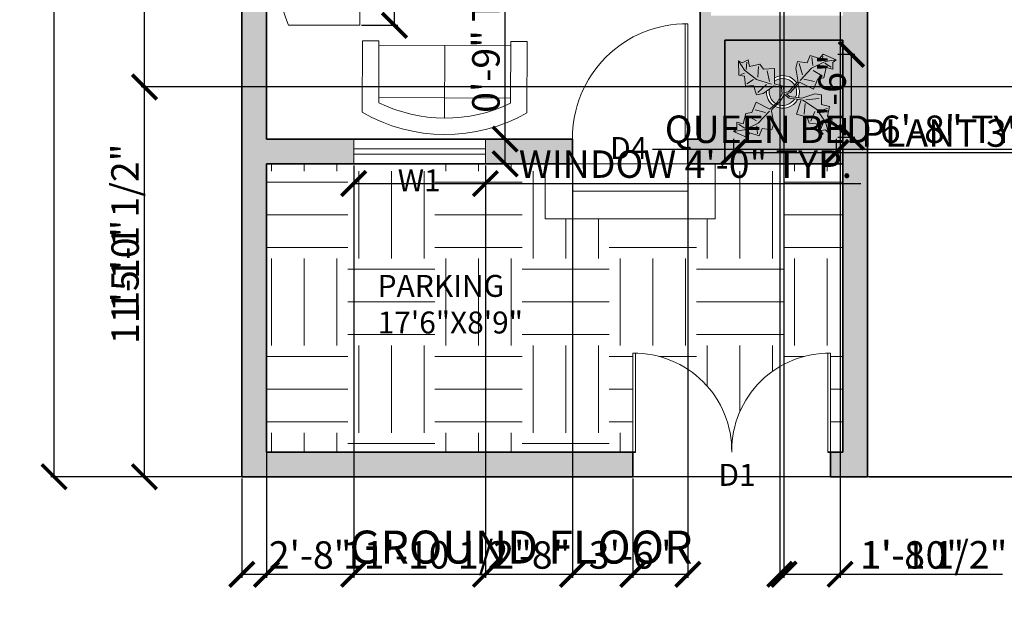
# Model space of a CAD drawing. Units: inches. Extents: x 2570 to 3313, y 1387 to 2106.
# Tile 1 of 5: x 2579 to 2938, y 1396 to 1607. Entities that reach past the tile are written whole.
import ezdxf

# ---------------------------------------------------------------- set-up
doc = ezdxf.new("R2010")
doc.units = ezdxf.units.IN
for name, color, linetype, lineweight in [('A-ANNO-DIMS', 7, 'Continuous', 18), ('DOORS', 195, 'Continuous', 18), ('furniture', 11, 'Continuous', 18), ('PLANT', 107, 'Continuous', 18), ('STAIRS', 13, 'Continuous', 18), ('WALLS', 20, 'Continuous', 35), ('WINDOWS', 15, 'Continuous', 18)]:
    doc.layers.add(name, color=color, linetype=linetype, lineweight=lineweight)
for name, color, linetype, lineweight, true_color in [('A-ANNO-TEXT', 143, 'Continuous', 18, 0x7aafdf), ('A-ANNO-TITL', 52, 'Continuous', 25, 0xc8c92d), ('A-AREA-IDEN', 143, 'Continuous', 18, 0x7aafdf), ('A-FLOR-PATT', 254, 'Continuous', 13, 0xcecce6), ('A-WALL-PATT', 30, 'Continuous', 13, 0xf26722), ('L-PLNT-PATT', 114, 'Continuous', 13, 0x139b48)]:
    doc.layers.add(name, color=color, linetype=linetype, lineweight=lineweight, true_color=true_color)
doc.styles.get("Standard").update_dxf_attribs({"font": 'arial.ttf'})
doc.dimstyles.new('ISO-25', dxfattribs={"dimtxt": 10, "dimasz": 9, "dimexe": 1.25, "dimexo": 0.625, "dimtad": 1, "dimdec": 0, "dimlunit": 3, "dimtxsty": 'Standard', "dimblk": 'ARCHTICK', "dimcen": 2.5, "dimadec": 0, "dimazin": 0, "dimtfac": 1, "dimtdec": 0, "dimtmove": 0, "dimatfit": 3, "dimfxl": 1, "dimarcsym": 0})

# ---------------------------------------------------------------- blocks, each defined once
blk = doc.blocks.new('Plant - Rubber or Philodendron')
for p, q in [((-16.2005, 11.4774), (-13.9899, 8.1064)), ((-16.2005, 11.4774), (-14.8639, 10.7964)), ((-16.0159, 6.3329), (-16.2005, 11.4774)), ((-14.8639, 10.7964), (-12.6195, 11.8975)), ((-13.3174, 8.325), (-13.0735, 11.0065)), ((-12.6195, 11.8975), (-12.1909, 9.4345)), ((4.6914, 8.8812), (5.3859, 11.2828)), ((5.3859, 11.2828), (8.8871, 10.7908)), ((8.8871, 10.7908), (9.9809, 13.4933)), ((9.9809, 13.4933), (13.3837, 12.301)), ((15.3859, 11.3055), (10.3916, 8.7942)), ((10.5828, 12.6946), (10.8893, 9.7953)), ((13.3837, 12.301), (14.68, 13.9039)), ((14.5816, 13.2037), (14.3848, 11.8033)), ((14.68, 13.9039), (19.3848, 11.8146)), ((19.3848, 11.8146), (15.3859, 11.3055)), ((19.3848, 11.8146), (18.1868, 10.9119)), ((18.1868, 10.9119), (18.1925, 8.4119)), ((-13.9899, 8.1064), (-9.5434, 4.7185)), ((-12.1909, 9.4345), (-8.3829, 10.3)), ((-8.8369, 9.409), (-9.0894, 5.6095)), ((-8.3829, 10.3), (-7.0549, 8.501)), ((-7.0549, 8.501), (-3.0284, 8.6941)), ((-4.8529, 4.012), (-5.7184, 7.82)), ((-3.0284, 8.6941), (-3.0709, 3.1041)), ((4.6914, 8.8812), (5.5014, 4.4831)), ((5.9878, 10.4842), (7.1971, 6.3869)), ((10.3916, 8.7942), (6.2847, 4.4028)), ((14.2977, 6.1031), (10.9934, 7.9956)), ((15.7909, 9.1065), (14.8995, 5.3044)), ((15.2875, 10.6053), (17.5907, 9.2105)), ((18.1925, 8.4119), (15.7909, 9.1065)), ((-14.0069, 5.8704), (-16.0159, 6.3329)), ((-15.3434, 6.5514), (-13.9984, 6.9884)), ((-13.5868, 2.2894), (-14.0069, 5.8704)), ((-13.1329, 3.1804), (-10.6614, 4.727)), ((-9.5434, 4.7185), (-4.1917, 2.9888)), ((2.1141, 0.2298), (5.4346, 3.9146)), ((6.1032, 3.6844), (2.8262, -0.031)), ((5.4346, 3.9146), (5.5014, 4.4831)), ((11.1089, 1.1958), (6.1032, 3.6844)), ((7.7005, 4.8881), (11.5025, 3.9967)), ((12.7005, 4.8994), (11.1089, 1.1958)), ((14.8995, 5.3044), (12.7005, 4.8994)), ((-10.6784, 2.491), (-13.5868, 2.2894)), ((-9.5858, -0.8715), (-10.6784, 2.491)), ((-9.1318, 0.0195), (-5.9793, 2.9025)), ((-7.1228, -0.443), (-3.5248, 2.2131)), ((-3.5248, 2.2131), (-3.3011, 2.4355)), ((-3.3011, 2.4355), (-0.5306, 1.7947)), ((-3.0709, 3.1041), (0.0797, 2.3163)), ((-0.5306, 1.7947), (-0.2255, -0.5527)), ((-0.5306, 1.7947), (-0.5306, 1.7947)), ((0.0797, 2.3163), (0.4866, -0.031)), ((0.4866, -0.031), (2.1141, 0.2298)), ((-11.3237, -7.2629), (-9.7321, -3.5593)), ((-9.7321, -3.5593), (-4.7264, -6.0479)), ((-7.1228, -0.443), (-9.5858, -0.8715)), ((-4.0579, -6.2781), (-0.9375, -3.1608)), ((-2.019, -3.6148), (-0.2255, -0.5527)), ((-0.9375, -3.1608), (0.5883, -0.8135)), ((0.5883, -0.8135), (2.2447, -2.0916)), ((2.8262, -0.031), (1.3003, -0.5527)), ((1.3003, -0.5527), (2.4193, -1.4655)), ((2.2447, -2.0916), (6.7108, -2.6626)), ((2.4193, -1.4655), (6.895, -2.1175)), ((4.943, -7.9659), (6.7108, -2.6626)), ((11.6605, -0.5413), (6.895, -2.1175)), ((12.3677, -6.1981), (7.219, -2.6772)), ((8.3544, -2.7453), (13.1973, -2.1704)), ((11.6605, -0.5413), (14.1354, -0.8948)), ((14.1354, -0.8948), (14.1354, -4.4304)), ((-6.3237, -7.2516), (-10.1257, -6.3602)), ((-9.0148, -11.1577), (-4.9047, -6.8122)), ((-2.019, -3.6148), (-4.7264, -6.0479)), ((-4.1246, -6.8466), (-4.0579, -6.2781)), ((-3.3146, -11.2447), (-4.1246, -6.8466)), ((8.125, -4.0768), (7.7715, -7.9659)), ((10.2463, -10.4408), (11.6605, -6.9053)), ((15.5496, -10.7943), (12.3677, -6.1981)), ((16.2567, -5.8446), (13.4283, -6.5517)), ((14.1354, -4.4304), (16.9638, -5.1375)), ((16.9638, -5.1375), (16.2567, -8.673)), ((-14.4141, -11.4699), (-13.5228, -7.6679)), ((-13.5228, -7.6679), (-11.3237, -7.2629)), ((-12.921, -8.4665), (-9.6166, -10.359)), ((-4.611, -12.8477), (-5.8203, -8.7504)), ((8.8321, -9.0266), (4.943, -7.9659)), ((9.5392, -11.1479), (8.8321, -9.0266)), ((17.3174, -9.7337), (15.9032, -9.7337)), ((16.2567, -8.673), (18.0245, -9.7337)), ((18.0245, -9.7337), (16.6103, -14.6834)), ((-18.008, -14.1781), (-16.8101, -13.2754)), ((-18.008, -14.1781), (-14.0091, -13.669)), ((-13.3032, -16.2674), (-18.008, -14.1781)), ((-16.8157, -10.7754), (-14.4141, -11.4699)), ((-16.8101, -13.2754), (-16.8157, -10.7754)), ((-13.9107, -12.9688), (-16.2139, -11.574)), ((-14.0091, -13.669), (-9.0148, -11.1577)), ((-13.2048, -15.5672), (-13.008, -14.1668)), ((-9.206, -15.0581), (-9.5126, -12.1588)), ((-7.5103, -13.1543), (-8.6042, -15.8568)), ((-4.0092, -13.6463), (-7.5103, -13.1543)), ((-3.3146, -11.2447), (-4.0092, -13.6463)), ((13.4283, -11.5015), (9.5392, -11.1479)), ((13.0748, -13.9763), (13.4283, -11.5015)), ((15.5496, -13.6228), (13.0748, -13.9763)), ((14.8425, -10.7943), (13.7819, -13.2692)), ((16.6103, -14.6834), (15.5496, -10.7943)), ((16.6103, -14.6834), (15.5496, -13.6228)), ((-12.0069, -14.6645), (-13.3032, -16.2674)), ((-8.6042, -15.8568), (-12.0069, -14.6645))]:
    blk.add_line(p, q)
for centre, radius, start, end in [((0, 0), 6.1275, 34.37569, 120.1028), ((-0.0601, -0.2075), 5.2461, 33.82192, 124.9414), ((0.0308, 0.1664), 6, 178.6147, 235.1169), ((0.0308, 0.1664), 5, 168.1647, 238.6725), ((-0.2664, 0.1682), 5.2775, 338.4094, 20.03007), ((-0.098, 0.1364), 6.1288, 341.2017, 26.09184), ((-0.0234, 0.3825), 6.1492, 242.5812, 331.2714), ((-0.1102, 0.4886), 5.2883, 247.3711, 327.472)]:
    blk.add_arc(centre, radius, start, end)
blk = doc.blocks.new('Sofa - Roundback 7 ft.')
for p, q in [((-12.00002, -32.4421), (-12.00003, -6.5971)), ((11.99997, -32.4421), (11.99998, -6.5971)), ((-36.000027, -34), (-36.000027, -11.4696)), ((-35.999844, -13.3819), (35.9998, -13.3819)), ((35.99998, -34), (35.99998, -11.4696)), ((-36.000027, -32.4421), (35.99998, -32.4421))]:
    blk.add_line(p, q)
for points in [[(-36.000027, -34), (-42.000027, -34), (-42.000027, -8)], [(41.99998, -8), (41.99998, -34), (35.99998, -34)]]:
    blk.add_lwpolyline(points)
for centre, radius, start, end in [((0, -114.25), 114.25, 68.43141, 111.5686), ((-0.00001, -127.1968), 121.1968, 72.72033, 107.2797)]:
    blk.add_arc(centre, radius, start, end)
blk = doc.blocks.new('Sofa - Roundback Loveseat 5 ft.')
for p, q in [((0, -32.44198), (0, -5.99998)), ((-24, -33.99998), (-24, -11.46958)), ((-23.9998, -13.38178), (23.99986, -13.38178)), ((24.00004, -33.99998), (24.00004, -11.46958)), ((-24, -32.44198), (24.00004, -32.44198))]:
    blk.add_line(p, q)
for points in [[(-24, -33.99998), (-30, -33.99998), (-30, -7.99998)], [(30.00004, -7.99998), (30.00004, -33.99998), (24.00004, -33.99998)]]:
    blk.add_lwpolyline(points)
for centre, radius, start, end in [((0, -60.24998), 60.24998, 60.13715, 119.8628), ((0, -61.38438), 55.38444, 64.32083, 115.6792)]:
    blk.add_arc(centre, radius, start, end)
blk = doc.blocks.new('_ArchTick')
at = {"color": 0, "linetype": 'ByBlock', "const_width": 0.15}
blk.add_lwpolyline([(-0.5, -0.5), (0.5, 0.5)], dxfattribs=at)
blk = doc.blocks.new('*D20')
at = {"layer": 'A-ANNO-DIMS', "color": 0, "lineweight": -2, "transparency": 16777216}
for p, q in [((2659.53, 2040.49), (2590.49, 2040.49)), ((2591.74, 1440.49), (2591.74, 2040.49)), ((2659.53, 1440.49), (2590.49, 1440.49))]:
    blk.add_line(p, q, dxfattribs=at)
at = {"layer": 'Defpoints', "color": 0, "transparency": 16777216}
for p in [(2591.74, 2040.49), (2660.15, 2040.49), (2660.15, 1440.49)]:
    blk.add_point(p, dxfattribs=at)
at = {"layer": 'A-ANNO-DIMS', "color": 0, "lineweight": -2, "transparency": 16777216, "xscale": 9, "yscale": 9, "zscale": 9}
for p, rotation in [((2591.74, 2040.49), 90), ((2591.74, 1440.49), 270)]:
    blk.add_blockref('_ArchTick', p, dxfattribs=dict(at, rotation=rotation))
at = {"layer": 'A-ANNO-DIMS', "color": 0, "transparency": 16777216, "insert": (2586.01, 1740.49), "char_height": 10, "attachment_point": 5, "rotation": 90}
blk.add_mtext("50'", dxfattribs=at)
blk = doc.blocks.new('WIN-48IN')
for p, q in [((-48, 0), (-48, -9)), ((0, 0), (0, -9)), ((0, -3.5), (-48, -3.5)), ((0, -5.5), (-48, -5.5))]:
    blk.add_line(p, q)
blk = doc.blocks.new('*D37')
at = {"layer": 'A-ANNO-DIMS', "color": 0, "lineweight": -2, "transparency": 16777216}
for p, q in [((2700.9, 1553.86), (2700.9, 1546.04)), ((2748.9, 1553.86), (2748.9, 1546.04)), ((2700.9, 1547.29), (2748.9, 1547.29)), ((2748.9, 1547.29), (2885.7, 1547.29))]:
    blk.add_line(p, q, dxfattribs=at)
at = {"layer": 'Defpoints', "color": 0, "transparency": 16777216}
for p in [(2700.9, 1554.49), (2748.9, 1554.49), (2748.9, 1547.29)]:
    blk.add_point(p, dxfattribs=at)
at = {"layer": 'A-ANNO-DIMS', "color": 0, "lineweight": -2, "transparency": 16777216, "xscale": 9, "yscale": 9, "zscale": 9, "rotation": 180}
blk.add_blockref('_ArchTick', (2700.9, 1547.29), dxfattribs=at)
at = {"layer": 'A-ANNO-DIMS', "color": 0, "lineweight": -2, "transparency": 16777216, "xscale": 9, "yscale": 9, "zscale": 9}
blk.add_blockref('_ArchTick', (2748.9, 1547.29), dxfattribs=at)
at = {"layer": 'A-ANNO-DIMS', "color": 0, "transparency": 16777216, "insert": (2821.8, 1553.09), "char_height": 10, "attachment_point": 5}
blk.add_mtext('WINDOW 4\'-0" TYP.', dxfattribs=at)
blk = doc.blocks.new('*D38')
at = {"layer": 'A-ANNO-DIMS', "color": 0, "lineweight": -2, "transparency": 16777216}
for p, q in [((2756.1, 1563.49), (2756.1, 1634.69)), ((2749.53, 1563.49), (2757.35, 1563.49)), ((2756.1, 1554.49), (2756.1, 1563.49)), ((2749.53, 1554.49), (2757.35, 1554.49))]:
    blk.add_line(p, q, dxfattribs=at)
at = {"layer": 'Defpoints', "color": 0, "transparency": 16777216}
for p in [(2748.9, 1563.49), (2756.1, 1563.49), (2748.9, 1554.49)]:
    blk.add_point(p, dxfattribs=at)
at = {"layer": 'A-ANNO-DIMS', "color": 0, "lineweight": -2, "transparency": 16777216, "xscale": 9, "yscale": 9, "zscale": 9}
for p, rotation in [((2756.1, 1563.49), 90), ((2756.1, 1554.49), 270)]:
    blk.add_blockref('_ArchTick', p, dxfattribs=dict(at, rotation=rotation))
at = {"layer": 'A-ANNO-DIMS', "color": 0, "transparency": 16777216, "insert": (2750.37, 1603.59), "char_height": 10, "attachment_point": 5, "rotation": 90}
blk.add_mtext('0\'-9" TYP.', dxfattribs=at)
blk = doc.blocks.new('*D49')
at = {"layer": 'A-ANNO-DIMS', "color": 0, "lineweight": -2, "transparency": 16777216}
for p, q in [((2967.16, 1571.06), (2967.16, 1558.44)), ((3047.16, 1571.06), (3047.16, 1558.44)), ((2967.16, 1559.69), (2809.81, 1559.69)), ((3047.16, 1559.69), (2967.16, 1559.69))]:
    blk.add_line(p, q, dxfattribs=at)
at = {"layer": 'Defpoints', "color": 0, "transparency": 16777216}
for p in [(2967.16, 1571.69), (3047.16, 1571.69), (2967.16, 1559.69)]:
    blk.add_point(p, dxfattribs=at)
at = {"layer": 'A-ANNO-DIMS', "color": 0, "lineweight": -2, "transparency": 16777216, "xscale": 9, "yscale": 9, "zscale": 9, "rotation": 180}
blk.add_blockref('_ArchTick', (2967.16, 1559.69), dxfattribs=at)
at = {"layer": 'A-ANNO-DIMS', "color": 0, "lineweight": -2, "transparency": 16777216, "xscale": 9, "yscale": 9, "zscale": 9}
blk.add_blockref('_ArchTick', (3047.16, 1559.69), dxfattribs=at)
at = {"layer": 'A-ANNO-DIMS', "color": 0, "transparency": 16777216, "insert": (2883.99, 1565.79), "char_height": 10, "attachment_point": 5}
blk.add_mtext('QUEEN BED 6\'-8" TYP.', dxfattribs=at)
blk = doc.blocks.new('*D50')
at = {"layer": 'A-ANNO-DIMS', "color": 0, "lineweight": -2, "transparency": 16777216}
for p, q in [((2955.16, 1631.69), (2955.16, 1702.89)), ((2966.54, 1631.69), (2953.91, 1631.69)), ((2955.16, 1571.69), (2955.16, 1631.69)), ((2966.54, 1571.69), (2953.91, 1571.69))]:
    blk.add_line(p, q, dxfattribs=at)
at = {"layer": 'Defpoints', "color": 0, "transparency": 16777216}
for p in [(2955.16, 1631.69), (2967.16, 1631.69), (2967.16, 1571.69)]:
    blk.add_point(p, dxfattribs=at)
at = {"layer": 'A-ANNO-DIMS', "color": 0, "lineweight": -2, "transparency": 16777216, "xscale": 9, "yscale": 9, "zscale": 9}
for p, rotation in [((2955.16, 1631.69), 90), ((2955.16, 1571.69), 270)]:
    blk.add_blockref('_ArchTick', p, dxfattribs=dict(at, rotation=rotation))
at = {"layer": 'A-ANNO-DIMS', "color": 0, "transparency": 16777216, "insert": (2949.43, 1671.79), "char_height": 10, "attachment_point": 5, "rotation": 90}
blk.add_mtext('5\'-0" TYP.', dxfattribs=at)
blk = doc.blocks.new('*D55')
at = {"layer": 'A-ANNO-DIMS', "color": 0, "lineweight": -2, "transparency": 16777216}
for p, q in [((2839.28, 1563.6), (2839.28, 1557.37)), ((2876.67, 1563.6), (2876.67, 1557.37)), ((2839.28, 1558.62), (2876.67, 1558.62)), ((2876.67, 1558.62), (2985.22, 1558.62))]:
    blk.add_line(p, q, dxfattribs=at)
at = {"layer": 'Defpoints', "color": 0, "transparency": 16777216}
for p in [(2839.28, 1564.23), (2876.67, 1564.23), (2876.67, 1558.62)]:
    blk.add_point(p, dxfattribs=at)
at = {"layer": 'A-ANNO-DIMS', "color": 0, "lineweight": -2, "transparency": 16777216, "xscale": 9, "yscale": 9, "zscale": 9, "rotation": 180}
blk.add_blockref('_ArchTick', (2839.28, 1558.62), dxfattribs=at)
at = {"layer": 'A-ANNO-DIMS', "color": 0, "lineweight": -2, "transparency": 16777216, "xscale": 9, "yscale": 9, "zscale": 9}
blk.add_blockref('_ArchTick', (2876.67, 1558.62), dxfattribs=at)
at = {"layer": 'A-ANNO-DIMS', "color": 0, "transparency": 16777216, "insert": (2935.45, 1564.42), "char_height": 10, "attachment_point": 5}
blk.add_mtext('PLANT 3\'-1 1/2"', dxfattribs=at)
blk = doc.blocks.new('*D56')
at = {"layer": 'A-ANNO-DIMS', "color": 0, "lineweight": -2, "transparency": 16777216}
for p, q in [((2877.3, 1594.4), (2883.53, 1594.4)), ((2882.28, 1564.23), (2882.28, 1594.4)), ((2877.3, 1564.23), (2883.53, 1564.23))]:
    blk.add_line(p, q, dxfattribs=at)
at = {"layer": 'Defpoints', "color": 0, "transparency": 16777216}
for p in [(2876.67, 1594.4), (2882.28, 1594.4), (2876.67, 1564.23)]:
    blk.add_point(p, dxfattribs=at)
at = {"layer": 'A-ANNO-DIMS', "color": 0, "lineweight": -2, "transparency": 16777216, "xscale": 9, "yscale": 9, "zscale": 9}
for p, rotation in [((2882.28, 1594.4), 90), ((2882.28, 1564.23), 270)]:
    blk.add_blockref('_ArchTick', p, dxfattribs=dict(at, rotation=rotation))
at = {"layer": 'A-ANNO-DIMS', "color": 0, "transparency": 16777216, "insert": (2876.55, 1579.31), "char_height": 10, "attachment_point": 5, "rotation": 90}
blk.add_mtext('2\'-6"', dxfattribs=at)
blk = doc.blocks.new('*D59')
at = {"layer": 'A-ANNO-DIMS', "color": 0, "lineweight": -2, "transparency": 16777216}
for p, q in [((2703.78, 1688.95), (2717, 1688.95)), ((2715.75, 1604.95), (2715.75, 1688.95)), ((2703.78, 1604.95), (2717, 1604.95))]:
    blk.add_line(p, q, dxfattribs=at)
at = {"layer": 'Defpoints', "color": 0, "transparency": 16777216}
for p in [(2703.15, 1688.95), (2715.75, 1688.95), (2703.15, 1604.95)]:
    blk.add_point(p, dxfattribs=at)
at = {"layer": 'A-ANNO-DIMS', "color": 0, "lineweight": -2, "transparency": 16777216, "xscale": 9, "yscale": 9, "zscale": 9}
for p, rotation in [((2715.75, 1688.95), 90), ((2715.75, 1604.95), 270)]:
    blk.add_blockref('_ArchTick', p, dxfattribs=dict(at, rotation=rotation))
at = {"layer": 'A-ANNO-DIMS', "color": 0, "transparency": 16777216, "insert": (2709.95, 1646.95), "char_height": 10, "attachment_point": 5, "rotation": 90}
blk.add_mtext('SOFA 7\'-0"', dxfattribs=at)
blk = doc.blocks.new('*D64')
at = {"layer": 'A-ANNO-DIMS', "color": 0, "lineweight": -2, "transparency": 16777216}
for p, q in [((2660.15, 1439.86), (2660.15, 1403.74)), ((2802.65, 1439.86), (2802.65, 1403.74)), ((2660.15, 1404.99), (2802.65, 1404.99))]:
    blk.add_line(p, q, dxfattribs=at)
at = {"layer": 'Defpoints', "color": 0, "transparency": 16777216}
for p in [(2660.15, 1440.49), (2802.65, 1440.49), (2802.65, 1404.99)]:
    blk.add_point(p, dxfattribs=at)
at = {"layer": 'A-ANNO-DIMS', "color": 0, "lineweight": -2, "transparency": 16777216, "xscale": 9, "yscale": 9, "zscale": 9, "rotation": 180}
blk.add_blockref('_ArchTick', (2660.15, 1404.99), dxfattribs=at)
at = {"layer": 'A-ANNO-DIMS', "color": 0, "lineweight": -2, "transparency": 16777216, "xscale": 9, "yscale": 9, "zscale": 9}
blk.add_blockref('_ArchTick', (2802.65, 1404.99), dxfattribs=at)
at = {"layer": 'A-ANNO-DIMS', "color": 0, "transparency": 16777216, "insert": (2731.4, 1410.78), "char_height": 10, "attachment_point": 5}
blk.add_mtext('11\'-10 1/2"', dxfattribs=at)
blk = doc.blocks.new('*D68')
at = {"layer": 'A-ANNO-DIMS', "color": 0, "lineweight": -2, "transparency": 16777216}
for p, q in [((2659.53, 1621.99), (2623.4, 1621.99)), ((2624.65, 1440.49), (2624.65, 1621.99)), ((2659.53, 1440.49), (2623.4, 1440.49))]:
    blk.add_line(p, q, dxfattribs=at)
at = {"layer": 'Defpoints', "color": 0, "transparency": 16777216}
for p in [(2624.65, 1621.99), (2660.15, 1621.99), (2660.15, 1440.49)]:
    blk.add_point(p, dxfattribs=at)
at = {"layer": 'A-ANNO-DIMS', "color": 0, "lineweight": -2, "transparency": 16777216, "xscale": 9, "yscale": 9, "zscale": 9}
for p, rotation in [((2624.65, 1621.99), 90), ((2624.65, 1440.49), 270)]:
    blk.add_blockref('_ArchTick', p, dxfattribs=dict(at, rotation=rotation))
at = {"layer": 'A-ANNO-DIMS', "color": 0, "transparency": 16777216, "insert": (2618.86, 1531.24), "char_height": 10, "attachment_point": 5, "rotation": 90}
blk.add_mtext('15\'-1 1/2"', dxfattribs=at)
blk = doc.blocks.new('*D69')
at = {"layer": 'A-ANNO-DIMS', "color": 0, "lineweight": -2, "transparency": 16777216}
for p, q in [((2957.54, 1582.49), (2623.4, 1582.49)), ((2624.65, 1440.49), (2624.65, 1582.49)), ((2957.54, 1440.49), (2623.4, 1440.49))]:
    blk.add_line(p, q, dxfattribs=at)
at = {"layer": 'Defpoints', "color": 0, "transparency": 16777216}
for p in [(2624.65, 1582.49), (2958.16, 1582.49), (2958.16, 1440.49)]:
    blk.add_point(p, dxfattribs=at)
at = {"layer": 'A-ANNO-DIMS', "color": 0, "lineweight": -2, "transparency": 16777216, "xscale": 9, "yscale": 9, "zscale": 9}
for p, rotation in [((2624.65, 1582.49), 90), ((2624.65, 1440.49), 270)]:
    blk.add_blockref('_ArchTick', p, dxfattribs=dict(at, rotation=rotation))
at = {"layer": 'A-ANNO-DIMS', "color": 0, "transparency": 16777216, "insert": (2618.92, 1511.49), "char_height": 10, "attachment_point": 5, "rotation": 90}
blk.add_mtext('11\'-10"', dxfattribs=at)
blk = doc.blocks.new('*D72')
at = {"layer": 'A-ANNO-DIMS', "color": 0, "lineweight": -2, "transparency": 16777216}
for p, q in [((2780.65, 1553.86), (2780.65, 1403.74)), ((2822.65, 1553.86), (2822.65, 1403.74)), ((2780.65, 1404.99), (2822.65, 1404.99))]:
    blk.add_line(p, q, dxfattribs=at)
at = {"layer": 'Defpoints', "color": 0, "transparency": 16777216}
for p in [(2780.65, 1554.49), (2822.65, 1554.49), (2822.65, 1404.99)]:
    blk.add_point(p, dxfattribs=at)
at = {"layer": 'A-ANNO-DIMS', "color": 0, "lineweight": -2, "transparency": 16777216, "xscale": 9, "yscale": 9, "zscale": 9, "rotation": 180}
blk.add_blockref('_ArchTick', (2780.65, 1404.99), dxfattribs=at)
at = {"layer": 'A-ANNO-DIMS', "color": 0, "lineweight": -2, "transparency": 16777216, "xscale": 9, "yscale": 9, "zscale": 9}
blk.add_blockref('_ArchTick', (2822.65, 1404.99), dxfattribs=at)
at = {"layer": 'A-ANNO-DIMS', "color": 0, "transparency": 16777216, "insert": (2801.65, 1410.72), "char_height": 10, "attachment_point": 5}
blk.add_mtext('3\'-6"', dxfattribs=at)
blk = doc.blocks.new('*D73')
at = {"layer": 'A-ANNO-DIMS', "color": 0, "lineweight": -2, "transparency": 16777216}
for p, q in [((2669.15, 1553.86), (2669.15, 1403.74)), ((2700.9, 1553.86), (2700.9, 1403.74)), ((2669.15, 1404.99), (2700.9, 1404.99))]:
    blk.add_line(p, q, dxfattribs=at)
at = {"layer": 'Defpoints', "color": 0, "transparency": 16777216}
for p in [(2669.15, 1554.49), (2700.9, 1554.49), (2700.9, 1404.99)]:
    blk.add_point(p, dxfattribs=at)
at = {"layer": 'A-ANNO-DIMS', "color": 0, "lineweight": -2, "transparency": 16777216, "xscale": 9, "yscale": 9, "zscale": 9, "rotation": 180}
blk.add_blockref('_ArchTick', (2669.15, 1404.99), dxfattribs=at)
at = {"layer": 'A-ANNO-DIMS', "color": 0, "lineweight": -2, "transparency": 16777216, "xscale": 9, "yscale": 9, "zscale": 9}
blk.add_blockref('_ArchTick', (2700.9, 1404.99), dxfattribs=at)
at = {"layer": 'A-ANNO-DIMS', "color": 0, "transparency": 16777216, "insert": (2685.03, 1410.72), "char_height": 10, "attachment_point": 5}
blk.add_mtext('2\'-8"', dxfattribs=at)
blk = doc.blocks.new('*D74')
at = {"layer": 'A-ANNO-DIMS', "color": 0, "lineweight": -2, "transparency": 16777216}
for p, q in [((2748.9, 1553.86), (2748.9, 1403.74)), ((2780.65, 1553.86), (2780.65, 1403.74)), ((2748.9, 1404.99), (2780.65, 1404.99))]:
    blk.add_line(p, q, dxfattribs=at)
at = {"layer": 'Defpoints', "color": 0, "transparency": 16777216}
for p in [(2748.9, 1554.49), (2780.65, 1554.49), (2780.65, 1404.99)]:
    blk.add_point(p, dxfattribs=at)
at = {"layer": 'A-ANNO-DIMS', "color": 0, "lineweight": -2, "transparency": 16777216, "xscale": 9, "yscale": 9, "zscale": 9, "rotation": 180}
blk.add_blockref('_ArchTick', (2748.9, 1404.99), dxfattribs=at)
at = {"layer": 'A-ANNO-DIMS', "color": 0, "lineweight": -2, "transparency": 16777216, "xscale": 9, "yscale": 9, "zscale": 9}
blk.add_blockref('_ArchTick', (2780.65, 1404.99), dxfattribs=at)
at = {"layer": 'A-ANNO-DIMS', "color": 0, "transparency": 16777216, "insert": (2764.78, 1410.72), "char_height": 10, "attachment_point": 5}
blk.add_mtext('2\'-8"', dxfattribs=at)
blk = doc.blocks.new('*D76')
at = {"layer": 'A-ANNO-DIMS', "color": 0, "lineweight": -2, "transparency": 16777216}
for p, q in [((2888.78, 1633.4), (3222.91, 1633.4)), ((3221.66, 1440.49), (3221.66, 1633.4)), ((2888.78, 1440.49), (3222.91, 1440.49))]:
    blk.add_line(p, q, dxfattribs=at)
at = {"layer": 'Defpoints', "color": 0, "transparency": 16777216}
for p in [(2888.15, 1633.4), (3221.66, 1633.4), (2888.15, 1440.49)]:
    blk.add_point(p, dxfattribs=at)
at = {"layer": 'A-ANNO-DIMS', "color": 0, "lineweight": -2, "transparency": 16777216, "xscale": 9, "yscale": 9, "zscale": 9}
for p, rotation in [((3221.66, 1633.4), 90), ((3221.66, 1440.49), 270)]:
    blk.add_blockref('_ArchTick', p, dxfattribs=dict(at, rotation=rotation))
at = {"layer": 'A-ANNO-DIMS', "color": 0, "transparency": 16777216, "insert": (3215.93, 1536.94), "char_height": 10, "attachment_point": 5, "rotation": 90}
blk.add_mtext('16\'-1"', dxfattribs=at)
blk = doc.blocks.new('*D81')
at = {"layer": 'A-ANNO-DIMS', "color": 0, "lineweight": -2, "transparency": 16777216}
for p, q in [((2856.15, 1873.66), (2856.15, 1403.74)), ((2878.15, 1873.66), (2878.15, 1403.74)), ((2856.15, 1404.99), (2878.15, 1404.99)), ((2878.15, 1404.99), (2921.82, 1404.99))]:
    blk.add_line(p, q, dxfattribs=at)
at = {"layer": 'Defpoints', "color": 0, "transparency": 16777216}
for p in [(2856.15, 1874.28), (2878.15, 1874.28), (2878.15, 1404.99)]:
    blk.add_point(p, dxfattribs=at)
at = {"layer": 'A-ANNO-DIMS', "color": 0, "lineweight": -2, "transparency": 16777216, "xscale": 9, "yscale": 9, "zscale": 9, "rotation": 180}
blk.add_blockref('_ArchTick', (2856.15, 1404.99), dxfattribs=at)
at = {"layer": 'A-ANNO-DIMS', "color": 0, "lineweight": -2, "transparency": 16777216, "xscale": 9, "yscale": 9, "zscale": 9}
blk.add_blockref('_ArchTick', (2878.15, 1404.99), dxfattribs=at)
at = {"layer": 'A-ANNO-DIMS', "color": 0, "transparency": 16777216, "insert": (2904.48, 1410.72), "char_height": 10, "attachment_point": 5}
blk.add_mtext('1\'-10"', dxfattribs=at)
blk = doc.blocks.new('*D83')
at = {"layer": 'A-ANNO-DIMS', "color": 0, "lineweight": -2, "transparency": 16777216}
for p, q in [((2857.69, 1934.86), (2857.69, 1403.74)), ((2878.15, 1934.86), (2878.15, 1403.74)), ((2857.69, 1404.99), (2878.15, 1404.99)), ((2878.15, 1404.99), (2937.35, 1404.99))]:
    blk.add_line(p, q, dxfattribs=at)
at = {"layer": 'Defpoints', "color": 0, "transparency": 16777216}
for p in [(2857.69, 1935.48), (2878.15, 1935.48), (2878.15, 1404.99)]:
    blk.add_point(p, dxfattribs=at)
at = {"layer": 'A-ANNO-DIMS', "color": 0, "lineweight": -2, "transparency": 16777216, "xscale": 9, "yscale": 9, "zscale": 9, "rotation": 180}
blk.add_blockref('_ArchTick', (2857.69, 1404.99), dxfattribs=at)
at = {"layer": 'A-ANNO-DIMS', "color": 0, "lineweight": -2, "transparency": 16777216, "xscale": 9, "yscale": 9, "zscale": 9}
blk.add_blockref('_ArchTick', (2878.15, 1404.99), dxfattribs=at)
at = {"layer": 'A-ANNO-DIMS', "color": 0, "transparency": 16777216, "insert": (2912.25, 1410.78), "char_height": 10, "attachment_point": 5}
blk.add_mtext('1\'-8 1/2"', dxfattribs=at)

msp = doc.modelspace()

# ---------------------------------------------------------------- hatches: boundary and pattern name
at = {"layer": 'A-FLOR-PATT'}
h = msp.add_hatch(dxfattribs=at)
h.set_pattern_fill('EARTH', color=256, scale=5)
h.paths.add_polyline_path([(2802.65, 1485.49, -0.418286), (2838.66, 1450, -0.418345), (2874.65, 1485.49), (2874.65, 1449.49), (2879.15, 1449.49), (2879.15, 1554.49), (2832.65, 1554.49), (2832.65, 1534.49), (2770.65, 1534.49), (2770.65, 1554.49), (2669.15, 1554.49), (2669.15, 1449.49), (2802.65, 1449.49)])
h.paths.add_polyline_path([(2714.83, 1540.04), (2735.59, 1540.04), (2735.59, 1556.53), (2714.83, 1556.53)], flags=9)
h.paths.add_polyline_path([(2706.42, 1488.16), (2761.15, 1488.16), (2761.15, 1518.01), (2706.42, 1518.01)], flags=24)
at = {"layer": 'A-WALL-PATT'}
h = msp.add_hatch(color=256, dxfattribs=at)
h.dxf.hatch_style = 1
h.paths.add_polyline_path([(2888.15, 1871.99), (2879.15, 1871.99), (2879.15, 1817.49), (2851.15, 1817.49), (2851.15, 1813.49), (2879.15, 1813.49), (2879.15, 1657.4), (2888.15, 1657.4)])
h.paths.add_polyline_path([(2831.15, 1737.49), (2669.15, 1737.49), (2669.15, 1813.49), (2745.15, 1813.49), (2745.15, 1849.49), (2741.15, 1849.49), (2741.15, 1817.49), (2669.15, 1817.49), (2669.15, 1838.62), (2660.15, 1838.62), (2660.15, 1669.99), (2669.15, 1669.99), (2669.15, 1728.49), (2831.15, 1728.49)])
h.paths.add_polyline_path([(2669.15, 1621.99), (2660.15, 1621.99), (2660.15, 1440.49), (2802.65, 1440.49), (2802.65, 1449.49), (2669.15, 1449.49), (2669.15, 1554.49), (2700.9, 1554.49), (2700.9, 1563.49), (2669.15, 1563.49)])
h.paths.add_polyline_path([(2780.65, 1563.49), (2748.9, 1563.49), (2748.9, 1554.49), (2780.65, 1554.49)], flags=17)
h.paths.add_polyline_path([(2836.15, 1599.49), (2879.15, 1599.49), (2879.15, 1449.49), (2874.65, 1449.49), (2874.65, 1440.49), (2888.15, 1440.49), (2888.15, 1633.4), (2879.15, 1633.4), (2879.15, 1608.49), (2831.15, 1608.49), (2831.15, 1680.49), (2827.15, 1680.49), (2827.15, 1563.49), (2822.65, 1563.49), (2822.65, 1554.49), (2836.15, 1554.49)])
h.paths.add_polyline_path([(2793.15, 1962.49), (2821.15, 1962.49), (2821.15, 1971.49), (2793.15, 1971.49), (2793.15, 2031.49), (2818.15, 2031.49), (2818.15, 2040.49), (2747.15, 2040.49), (2747.15, 2031.49), (2789.15, 2031.49), (2789.15, 1887.49), (2785.15, 1887.49), (2785.15, 1879.49), (2789.15, 1879.49), (2789.15, 1817.49), (2789.15, 1813.49), (2793.15, 1813.49), (2821.15, 1813.49), (2821.15, 1817.49), (2793.15, 1817.49)])
h.paths.add_polyline_path([(2749.15, 1887.49), (2669.15, 1887.49), (2669.15, 2031.49), (2711.15, 2031.49), (2711.15, 2040.49), (2660.15, 2040.49), (2660.15, 1862.62), (2669.15, 1862.62), (2669.15, 1883.49), (2741.15, 1883.49), (2741.15, 1879.49), (2749.15, 1879.49)])
h.paths.add_polyline_path([(2888.15, 2040.49), (2854.15, 2040.49), (2854.15, 2031.49), (2879.15, 2031.49), (2879.15, 1971.49), (2877.15, 1971.49), (2877.15, 1962.49), (2879.15, 1962.49), (2879.15, 1907.99), (2888.15, 1907.99)])
h.paths.add_polyline_path([(2967.16, 2031.49), (3011.16, 2031.49), (3011.16, 2004.49), (3015.16, 2004.49), (3015.16, 2031.49), (3039.26, 2031.49), (3039.26, 2040.49), (2958.16, 2040.49), (2958.16, 1909.99), (2967.16, 1909.99), (2967.16, 1921.99), (2967.16, 1966.49)])
h.paths.add_polyline_path([(3186.16, 2040.49), (3063.26, 2040.49), (3063.26, 2031.49), (3087.16, 2031.49), (3087.16, 1970.49), (3015.16, 1970.49), (3015.16, 1974.49), (3011.16, 1974.49), (3011.16, 1966.49), (3177.16, 1966.49), (3177.16, 1817.49), (3172.66, 1817.49), (3172.66, 1813.49), (3177.16, 1813.49), (3177.16, 1721.56), (3186.16, 1721.56)])
h.paths.add_polyline_path([(3177.16, 2031.49), (3177.16, 1970.49), (3091.16, 1970.49), (3091.16, 2031.49)], flags=16)
h.paths.add_polyline_path([(2967.16, 1873.99), (2958.16, 1873.99), (2958.16, 1712.62), (2967.16, 1712.62), (2967.16, 1724.49), (3051.16, 1724.49), (3051.16, 1710.49), (3055.16, 1710.49), (3055.16, 1724.49), (3125.16, 1724.49), (3125.16, 1676.49), (3085.16, 1676.49), (3085.16, 1672.49), (3125.16, 1672.49), (3125.16, 1668.49), (3129.16, 1668.49), (3129.16, 1733.49), (2967.16, 1733.49), (2967.16, 1813.49), (3136.66, 1813.49), (3136.66, 1817.49), (2967.16, 1817.49)])
h.paths.add_polyline_path([(2967.16, 1672.49), (3055.16, 1672.49), (3055.16, 1680.49), (3051.16, 1680.49), (3051.16, 1676.49), (2967.16, 1676.49), (2967.16, 1688.62), (2958.16, 1688.62), (2958.16, 1618.49), (2967.16, 1618.49), (2967.16, 1631.69)])
h.paths.add_polyline_path([(3186.16, 1685.56), (3177.16, 1685.56), (3177.16, 1568.09), (3169.16, 1568.09), (3169.16, 1564.09), (3177.16, 1564.09), (3177.16, 1519.49), (3177.16, 1449.49), (3186.16, 1449.49)])
h.paths.add_polyline_path([(3129.16, 1564.09), (3129.16, 1632.49), (3125.16, 1632.49), (3125.16, 1528.49), (2967.16, 1528.49), (2967.16, 1582.49), (2958.16, 1582.49), (2958.16, 1449.49), (2967.16, 1449.49), (2967.16, 1519.49), (3129.16, 1519.49)])
h.paths.add_polyline_path([(3123.16, 1975.63), (3150.13, 1975.63), (3150.13, 1992.12), (3123.16, 1992.12)], flags=8)
h.paths.add_polyline_path([(3130.18, 1590.82), (3180.42, 1590.82), (3180.42, 1617.03), (3130.18, 1617.03)], flags=9)
at = {"layer": 'L-PLNT-PATT'}
h = msp.add_hatch(color=256, dxfattribs=at)
h.dxf.hatch_style = 1
h.paths.add_polyline_path([(2879.15, 1599.49), (2836.15, 1599.49), (2836.15, 1554.49), (2879.15, 1554.49)])
h.paths.add_polyline_path([(2866.83, 1569.35), (2866.12, 1571.47), (2862.23, 1572.53), (2864, 1577.83), (2862.7, 1578, -0.411662), (2854.43, 1575.42), (2853.23, 1574.22), (2853.17, 1573.65), (2853.98, 1569.25), (2853.28, 1566.85), (2849.78, 1567.34), (2848.69, 1564.64), (2845.28, 1565.83), (2843.99, 1564.23), (2839.28, 1566.32), (2840.48, 1567.22), (2840.47, 1569.72), (2842.88, 1569.03), (2843.77, 1572.83), (2845.97, 1573.23), (2847.56, 1576.94), (2852.56, 1574.45), (2853.95, 1575.7, -0.259564), (2851.33, 1580.91), (2850.17, 1580.05), (2847.7, 1579.62), (2846.61, 1582.99), (2843.7, 1582.79), (2843.28, 1586.37), (2841.27, 1586.83), (2841.09, 1591.97), (2842.43, 1591.29), (2844.67, 1592.39), (2845.1, 1589.93), (2848.91, 1590.8), (2850.23, 1589), (2854.26, 1589.19), (2854.24, 1585.81, -0.39032), (2862.33, 1583.98), (2862.72, 1584.41), (2862.79, 1584.98), (2861.98, 1589.38), (2862.68, 1591.78), (2866.18, 1591.29), (2867.27, 1593.99), (2870.67, 1592.8), (2871.97, 1594.4), (2876.67, 1592.31), (2875.48, 1591.41), (2875.48, 1588.91), (2873.08, 1589.6), (2872.19, 1585.8), (2869.99, 1585.4), (2868.4, 1581.69), (2863.39, 1584.18), (2862.68, 1583.37, -0.204816), (2862.96, 1578.56), (2864.18, 1578.38), (2868.95, 1579.95), (2871.43, 1579.6), (2871.43, 1576.07), (2874.25, 1575.36), (2873.55, 1571.82), (2875.31, 1570.76), (2873.9, 1565.81), (2872.84, 1566.87), (2870.36, 1566.52), (2870.72, 1568.99)], flags=16)
h = msp.add_hatch(color=256, dxfattribs=at)
h.dxf.hatch_style = 1
h.paths.add_polyline_path([(2854.23, 1584.59), (2854.22, 1583.6), (2857.37, 1582.81), (2857.78, 1580.47), (2859.4, 1580.73), (2861.61, 1583.17, 0.422141)], flags=17)
h.paths.add_polyline_path([(2857.06, 1579.94), (2856.76, 1582.29), (2853.99, 1582.93), (2853.76, 1582.71), (2852.44, 1581.73, 0.320154), (2854.72, 1576.39), (2855.27, 1576.88)], flags=17)
h.paths.add_polyline_path([(2861.63, 1578.14), (2859.53, 1578.4), (2857.88, 1579.68), (2856.35, 1577.34), (2855.13, 1576.11, 0.365185)], flags=17)
h.paths.add_polyline_path([(2861.95, 1582.55), (2860.12, 1580.47), (2858.59, 1579.94), (2859.71, 1579.03), (2861.92, 1578.71, 0.18838)], flags=17)
h.paths.add_polyline_path([(2873.08, 1589.6), (2875.48, 1588.91), (2875.48, 1591.41), (2876.67, 1592.31), (2871.97, 1594.4), (2870.67, 1592.8), (2867.27, 1593.99), (2866.18, 1591.29), (2862.68, 1591.78), (2861.98, 1589.38), (2862.79, 1584.98), (2862.72, 1584.41), (2859.4, 1580.73), (2857.78, 1580.47), (2857.37, 1582.81), (2854.22, 1583.6), (2854.23, 1584.59), (2854.26, 1589.19), (2850.23, 1589), (2848.91, 1590.8), (2845.1, 1589.93), (2844.67, 1592.39), (2842.43, 1591.29), (2841.09, 1591.97), (2841.27, 1586.83), (2843.28, 1586.37), (2843.7, 1582.79), (2846.61, 1582.99), (2847.7, 1579.62), (2850.17, 1580.05), (2853.76, 1582.71), (2853.99, 1582.93), (2856.76, 1582.29), (2857.06, 1579.94), (2855.27, 1576.88), (2854.72, 1576.39), (2852.56, 1574.45), (2847.56, 1576.94), (2845.97, 1573.23), (2843.77, 1572.83), (2842.88, 1569.03), (2840.47, 1569.72), (2840.48, 1567.22), (2839.28, 1566.32), (2843.99, 1564.23), (2845.28, 1565.83), (2848.69, 1564.64), (2849.78, 1567.34), (2853.28, 1566.85), (2853.98, 1569.25), (2853.17, 1573.65), (2853.23, 1574.22), (2856.35, 1577.34), (2857.88, 1579.68), (2859.53, 1578.4), (2861.63, 1578.14), (2864, 1577.83), (2862.23, 1572.53), (2866.12, 1571.47), (2866.83, 1569.35), (2870.72, 1568.99), (2870.36, 1566.52), (2872.84, 1566.87), (2873.9, 1565.81), (2875.31, 1570.76), (2873.55, 1571.82), (2874.25, 1575.36), (2871.43, 1576.07), (2871.43, 1579.6), (2868.95, 1579.95), (2864.18, 1578.38), (2859.71, 1579.03), (2858.59, 1579.94), (2860.12, 1580.47), (2863.39, 1584.18), (2868.4, 1581.69), (2869.99, 1585.4), (2872.19, 1585.8)])

# ---------------------------------------------------------------- linework, layer by layer
at = {"layer": 'DOORS'}
for p, q in [((2821.65, 1563.49), (2821.65, 1605.49)), ((2822.65, 1563.49), (2822.65, 1605.49)), ((2802.65, 1449.49), (2802.65, 1485.49)), ((2803.65, 1449.49), (2803.65, 1485.49)), ((2873.65, 1449.49), (2873.65, 1485.49)), ((2874.65, 1449.49), (2874.65, 1485.49))]:
    msp.add_line(p, q, dxfattribs=at)
for centre, radius, start, end in [((2822.15, 1563.99), 41.5, 89.3097, 180.6903), ((2803.15, 1449.99), 35.5, 359.1931, 90.8069), ((2874.15, 1450), 35.5, 89.1929, 180.0114)]:
    msp.add_arc(centre, radius, start, end, dxfattribs=at)
at = {"layer": 'STAIRS'}
for p, q in [((2770.65, 1534.49), (2770.65, 1554.49)), ((2822.65, 1554.49), (2780.65, 1554.49)), ((2780.65, 1544.49), (2780.65, 1554.49)), ((2822.65, 1544.49), (2822.65, 1554.49)), ((2832.65, 1534.49), (2832.65, 1554.49)), ((2822.65, 1544.49), (2780.65, 1544.49)), ((2832.65, 1534.49), (2770.65, 1534.49))]:
    msp.add_line(p, q, dxfattribs=at)
at = {"layer": 'WALLS'}
for p, q in [((2660.15, 1440.49), (2660.15, 2040.49)), ((2888.15, 2040.49), (2888.15, 1440.49)), ((2669.15, 1563.49), (2669.15, 1728.49)), ((2827.15, 1563.49), (2827.15, 1680.49)), ((2879.15, 1599.49), (2836.15, 1599.49)), ((2836.15, 1554.49), (2836.15, 1599.49)), ((2879.15, 1599.49), (2879.15, 1449.49)), ((2780.65, 1563.49), (2669.15, 1563.49)), ((2780.65, 1554.49), (2780.65, 1563.49)), ((2827.15, 1563.49), (2821.65, 1563.49)), ((2822.65, 1554.49), (2822.65, 1563.49)), ((2669.15, 1449.49), (2669.15, 1554.49)), ((2780.65, 1554.49), (2669.15, 1554.49)), ((2879.15, 1554.49), (2822.65, 1554.49)), ((2803.65, 1449.49), (2669.15, 1449.49)), ((2802.65, 1440.49), (2802.65, 1449.49)), ((2879.15, 1449.49), (2873.65, 1449.49)), ((2874.65, 1440.49), (2874.65, 1449.49)), ((2802.65, 1440.49), (2660.15, 1440.49)), ((2888.15, 1440.49), (2874.65, 1440.49))]:
    msp.add_line(p, q, dxfattribs=at)

# ---------------------------------------------------------------- block references
at = {"layer": 'furniture', "rotation": 90.00002216900027}
msp.add_blockref('Sofa - Roundback 7 ft.', (2669.15, 1646.95), dxfattribs=at)
at = {"layer": 'furniture', "xscale": -1, "rotation": 179.7583430135472}
msp.add_blockref('Sofa - Roundback Loveseat 5 ft.', (2733.97, 1565.17), dxfattribs=at)
at = {"layer": 'PLANT'}
msp.add_blockref('Plant - Rubber or Philodendron', (2857.29, 1580.5), dxfattribs=at)
at = {"layer": 'WINDOWS'}
msp.add_blockref('WIN-48IN', (2748.9, 1563.49), dxfattribs=at)

# ---------------------------------------------------------------- texts
at = {"layer": 'A-ANNO-TEXT', "char_height": 8, "attachment_point": 1}
for s, width, insert in [('D4', 13.0839, (2794.34, 1564.23)), ('W1', 13.4987, (2716.96, 1552.45)), ('D1', 60.8198, (2833.8, 1445.2))]:
    msp.add_mtext_dynamic_manual_height_columns(s, width=width, gutter_width=12.5, heights=[0], dxfattribs=dict(at, insert=insert))
at = {"layer": 'A-ANNO-TITL', "insert": (2699.37, 1420.89), "char_height": 12, "attachment_point": 1}
msp.add_mtext_dynamic_manual_height_columns('{\\fArial|b1|i0|c0|p34;GROUND FLOOR}', width=181.3713, gutter_width=12.5, heights=[0], dxfattribs=at)
at = {"layer": 'A-AREA-IDEN', "insert": (2709.63, 1514.03), "char_height": 8, "attachment_point": 1}
msp.add_mtext_dynamic_manual_height_columns('PARKING\\P17\'6"X8\'9"', width=60.8198, gutter_width=12.5, heights=[0], dxfattribs=at)

# ---------------------------------------------------------------- dimensions: what is measured, and where the dimension line sits
at = {"layer": 'A-ANNO-DIMS'}
for base, p1, p2, override, picture, middle in [((2591.74, 2040.49), (2660.15, 1440.49), (2660.15, 2040.49), {"dimclrd": 0, "dimclre": 0, "dimclrt": 0}, '*D20', (2586.01, 1740.49)), ((3221.66, 1633.4), (2888.15, 1440.49), (2888.15, 1633.4), {"dimdec": 1, "dimlfac": 1, "dimrnd": 0, "dimzin": 1, "dimdsep": 46, "dimlunit": 4, "dimfrac": 2}, '*D76', (3215.93, 1536.94)), ((2624.65, 1621.99), (2660.15, 1440.49), (2660.15, 1621.99), {"dimdec": 1, "dimlfac": 1, "dimrnd": 0, "dimzin": 1, "dimdsep": 46, "dimlunit": 4, "dimfrac": 2}, '*D68', (2618.86, 1531.24)), ((2882.28, 1594.4), (2876.67, 1564.23), (2876.67, 1594.4), {"dimdec": 1, "dimlfac": 1, "dimrnd": 0, "dimzin": 1, "dimdsep": 46, "dimlunit": 4, "dimfrac": 2}, '*D56', (2876.55, 1579.31)), ((2624.65, 1582.49), (2958.16, 1440.49), (2958.16, 1582.49), {"dimdec": 1, "dimlfac": 1, "dimrnd": 0, "dimzin": 1, "dimdsep": 46, "dimlunit": 4, "dimfrac": 2}, '*D69', (2618.92, 1511.49))]:
    dim = msp.add_linear_dim(base=base, p1=p1, p2=p2, angle=90, dimstyle='ISO-25', override=override, dxfattribs=at)
    dim.commit()
    dim.dimension.update_dxf_attribs({"geometry": picture, "text_midpoint": middle})
for base, p1, p2, picture, middle in [((2878.15, 1404.99), (2857.69, 1935.48), (2878.15, 1935.48), '*D83', (2912.25, 1410.78)), ((2878.15, 1404.99), (2856.15, 1874.28), (2878.15, 1874.28), '*D81', (2904.48, 1410.72)), ((2700.904541, 1404.988461), (2669.154541, 1554.488461), (2700.904541, 1554.488461), '*D73', (2685.029541, 1410.71919088)), ((2780.654541, 1404.988461), (2748.904541, 1554.488461), (2780.654541, 1554.488461), '*D74', (2764.779541, 1410.71919088)), ((2822.65, 1404.99), (2780.65, 1554.49), (2822.65, 1554.49), '*D72', (2801.65, 1410.72)), ((2802.65, 1404.99), (2660.15, 1440.49), (2802.65, 1440.49), '*D64', (2731.4, 1410.78))]:
    dim = msp.add_linear_dim(base=base, p1=p1, p2=p2, dimstyle='ISO-25', override={"dimdec": 1, "dimlfac": 1, "dimrnd": 0, "dimzin": 1, "dimdsep": 46, "dimlunit": 4, "dimfrac": 2}, dxfattribs=at)
    dim.commit()
    dim.dimension.update_dxf_attribs({"geometry": picture, "text_midpoint": middle})
for base, p1, p2, angle, text, picture, middle in [((2955.16, 1631.69), (2967.16, 1571.69), (2967.16, 1631.69), 90, '<> TYP.', '*D50', (2949.43, 1671.79)), ((2715.75, 1688.95), (2703.15, 1604.95), (2703.15, 1688.95), 90, 'SOFA <>', '*D59', (2709.95, 1646.95)), ((2756.1, 1563.49), (2748.9, 1554.49), (2748.9, 1563.49), 90, '<> TYP.', '*D38', (2750.37, 1603.59)), ((2967.16, 1559.69), (3047.16, 1571.69), (2967.16, 1571.69), 180, 'QUEEN BED <> TYP.', '*D49', (2883.99, 1565.79))]:
    dim = msp.add_linear_dim(base=base, p1=p1, p2=p2, angle=angle, text=text, dimstyle='ISO-25', override={"dimdec": 1, "dimlfac": 1, "dimrnd": 0, "dimzin": 1, "dimdsep": 46, "dimlunit": 4, "dimfrac": 2}, dxfattribs=at)
    dim.commit()
    dim.dimension.update_dxf_attribs({"geometry": picture, "text_midpoint": middle})
for base, p1, p2, text, picture, middle in [((2876.67, 1558.62), (2839.28, 1564.23), (2876.67, 1564.23), 'PLANT <>', '*D55', (2935.45, 1564.42)), ((2748.9, 1547.29), (2700.9, 1554.49), (2748.9, 1554.49), 'WINDOW <> TYP.', '*D37', (2821.8, 1553.09))]:
    dim = msp.add_linear_dim(base=base, p1=p1, p2=p2, text=text, dimstyle='ISO-25', override={"dimdec": 1, "dimlfac": 1, "dimrnd": 0, "dimzin": 1, "dimdsep": 46, "dimlunit": 4, "dimfrac": 2}, dxfattribs=at)
    dim.commit()
    dim.dimension.update_dxf_attribs({"geometry": picture, "text_midpoint": middle})

doc.saveas('drawing.dxf')
